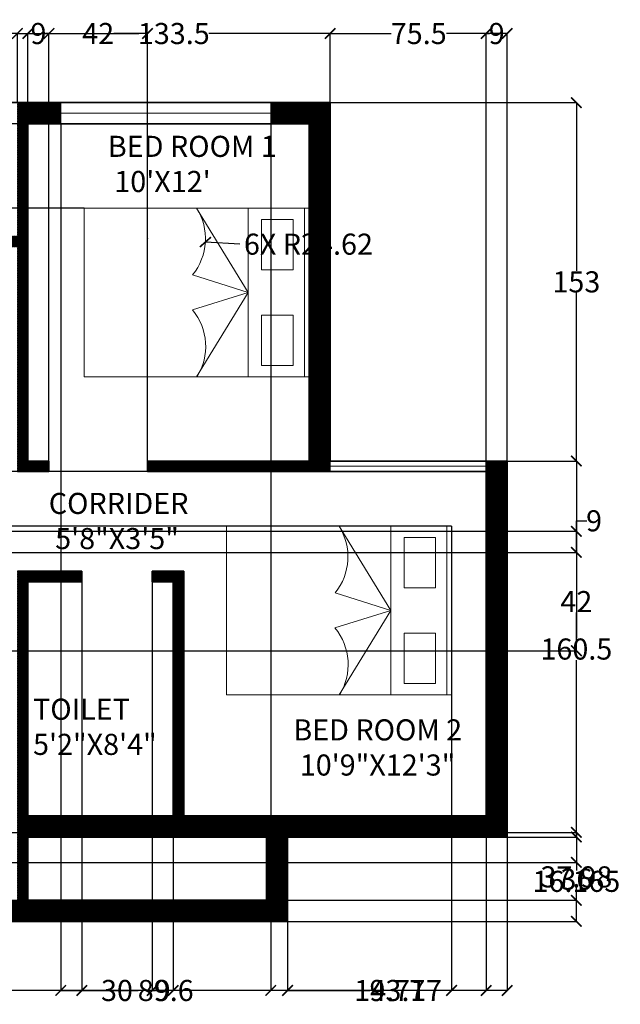
# Model space of a CAD drawing. Units: inches. Extents: x -9 to 675, y 146 to 566.
# Tile 4 of 4: x 418 to 675, y 146 to 566. Entities that reach past the tile are written whole.
import ezdxf

# ---------------------------------------------------------------- set-up
doc = ezdxf.new("R2010")
doc.units = ezdxf.units.IN
doc.header["$MEASUREMENT"] = 0
for name, color, linetype, lineweight in [('A-ANNO-DIMS', 2, 'Continuous', 18), ('A-AREA-IDEN', 7, 'Continuous', 18), ('A-FURN', 8, 'Continuous', 18), ('A-GLAZ', 4, 'Continuous', 18), ('A-WALL', 7, 'Continuous', 35), ('A-WALL-PATT', 252, 'Continuous', 13)]:
    doc.layers.add(name, color=color, linetype=linetype, lineweight=lineweight)
doc.styles.get("Standard").update_dxf_attribs({"font": 'arial.ttf'})
doc.dimstyles.get("Standard").update_dxf_attribs({"dimtxt": 9, "dimasz": 4.5, "dimexe": 0.18, "dimexo": 0.0625, "dimgap": 0.09, "dimtad": 0, "dimtih": 1, "dimtoh": 1, "dimdec": 1, "dimzin": 0, "dimdsep": 46, "dimlunit": 4, "dimtxsty": 'Standard', "dimblk": 'ARCHTICK', "dimcen": 0.09, "dimadec": 0, "dimazin": 0, "dimtfac": 1, "dimtdec": 1, "dimtofl": 0, "dimtmove": 0, "dimatfit": 3, "dimfxl": 1, "dimtolj": 1, "dimtzin": 0, "dimarcsym": 0})

# ---------------------------------------------------------------- blocks, each defined once
blk = doc.blocks.new('BED-DOUBLE-72X96')
for p, q in [((0, 0.1), (0, 72.1)), ((0, 72.1), (96, 72.1)), ((70, 36.1), (48, 72.1)), ((70, 72.1), (70, 0.1)), ((94, 72.1), (94, 0.1)), ((96, 72.1), (96, 0.1)), ((46.29, 43.57), (70, 36.1)), ((70, 36.1), (46.22, 28.65)), ((48, 0.1), (70, 36.1)), ((96, 0.1), (0, 0.1))]:
    blk.add_line(p, q)
for points in [[(89.14, 67.27), (89.14, 45.76), (75.68, 45.76), (75.68, 67.27)], [(89.14, 4.92), (89.14, 26.43), (75.68, 26.43), (75.68, 4.92)]]:
    blk.add_lwpolyline(points, close=True)
for centre, start, end in [((27.13, 59.03), 321.0858, 32.0518), ((27.23, 12.97), 328.2029, 39.5369)]:
    blk.add_arc(centre, 24.62, start, end)
blk = doc.blocks.new('_ArchTick')
at = {"color": 0, "linetype": 'ByBlock', "const_width": 0.15}
blk.add_lwpolyline([(-0.5, -0.5), (0.5, 0.5)], dxfattribs=at)
blk = doc.blocks.new('*D8')
at = {"layer": 'A-ANNO-DIMS', "color": 0, "lineweight": -2, "transparency": 16777216}
for p, q in [((626.3, 217.45), (626.3, 151.83)), ((39.3, 181.45), (39.3, 151.83)), ((39.3, 152.01), (322.77, 152.01)), ((626.3, 152.01), (342.83, 152.01))]:
    blk.add_line(p, q, dxfattribs=at)
at = {"layer": 'Defpoints', "color": 0, "transparency": 16777216}
for p in [(626.3, 217.51), (39.3, 181.51), (626.3, 152.01)]:
    blk.add_point(p, dxfattribs=at)
at = {"layer": 'A-ANNO-DIMS', "color": 0, "lineweight": -2, "transparency": 16777216, "xscale": 4.5, "yscale": 4.5, "zscale": 4.5, "rotation": 180}
blk.add_blockref('_ArchTick', (39.3, 152.01), dxfattribs=at)
at = {"layer": 'A-ANNO-DIMS', "color": 0, "lineweight": -2, "transparency": 16777216, "xscale": 4.5, "yscale": 4.5, "zscale": 4.5}
blk.add_blockref('_ArchTick', (626.3, 152.01), dxfattribs=at)
at = {"layer": 'A-ANNO-DIMS', "color": 0, "transparency": 16777216, "insert": (332.8, 152.01), "char_height": 9, "attachment_point": 5}
blk.add_mtext('\\A1;587', dxfattribs=at)
blk = doc.blocks.new('*D13')
at = {"layer": 'A-ANNO-DIMS', "color": 0, "lineweight": -2, "transparency": 16777216}
for p, q in [((286.8, 531.07), (286.8, 560.69)), ((286.8, 560.51), (337.17, 560.51)), ((417.3, 560.51), (366.94, 560.51)), ((417.3, 531.07), (417.3, 560.69))]:
    blk.add_line(p, q, dxfattribs=at)
at = {"layer": 'Defpoints', "color": 0, "transparency": 16777216}
for p in [(417.3, 560.51), (286.8, 531.01), (417.3, 531.01)]:
    blk.add_point(p, dxfattribs=at)
at = {"layer": 'A-ANNO-DIMS', "color": 0, "lineweight": -2, "transparency": 16777216, "xscale": 4.5, "yscale": 4.5, "zscale": 4.5, "rotation": 180}
blk.add_blockref('_ArchTick', (286.8, 560.51), dxfattribs=at)
at = {"layer": 'A-ANNO-DIMS', "color": 0, "lineweight": -2, "transparency": 16777216, "xscale": 4.5, "yscale": 4.5, "zscale": 4.5}
blk.add_blockref('_ArchTick', (417.3, 560.51), dxfattribs=at)
at = {"layer": 'A-ANNO-DIMS', "color": 0, "transparency": 16777216, "insert": (352.05, 560.51), "char_height": 9, "attachment_point": 5}
blk.add_mtext('\\A1;130.5', dxfattribs=at)
blk = doc.blocks.new('*D14')
at = {"layer": 'A-ANNO-DIMS', "color": 0, "lineweight": -2, "transparency": 16777216}
for p, q in [((417.3, 531.07), (417.3, 560.69)), ((417.3, 560.51), (469.17, 560.51)), ((550.8, 560.51), (498.94, 560.51)), ((550.8, 531.07), (550.8, 560.69))]:
    blk.add_line(p, q, dxfattribs=at)
at = {"layer": 'Defpoints', "color": 0, "transparency": 16777216}
for p in [(550.8, 560.51), (417.3, 531.01), (550.8, 531.01)]:
    blk.add_point(p, dxfattribs=at)
at = {"layer": 'A-ANNO-DIMS', "color": 0, "lineweight": -2, "transparency": 16777216, "xscale": 4.5, "yscale": 4.5, "zscale": 4.5, "rotation": 180}
blk.add_blockref('_ArchTick', (417.3, 560.51), dxfattribs=at)
at = {"layer": 'A-ANNO-DIMS', "color": 0, "lineweight": -2, "transparency": 16777216, "xscale": 4.5, "yscale": 4.5, "zscale": 4.5}
blk.add_blockref('_ArchTick', (550.8, 560.51), dxfattribs=at)
at = {"layer": 'A-ANNO-DIMS', "color": 0, "transparency": 16777216, "insert": (484.05, 560.51), "char_height": 9, "attachment_point": 5}
blk.add_mtext('\\A1;133.5', dxfattribs=at)
blk = doc.blocks.new('*D15')
at = {"layer": 'A-ANNO-DIMS', "color": 0, "lineweight": -2, "transparency": 16777216}
for p, q in [((550.8, 378.07), (550.8, 560.69)), ((550.8, 560.51), (576.78, 560.51)), ((626.3, 560.51), (600.33, 560.51)), ((626.3, 378.07), (626.3, 560.69))]:
    blk.add_line(p, q, dxfattribs=at)
at = {"layer": 'Defpoints', "color": 0, "transparency": 16777216}
for p in [(626.3, 560.51), (550.8, 378.01), (626.3, 378.01)]:
    blk.add_point(p, dxfattribs=at)
at = {"layer": 'A-ANNO-DIMS', "color": 0, "lineweight": -2, "transparency": 16777216, "xscale": 4.5, "yscale": 4.5, "zscale": 4.5, "rotation": 180}
blk.add_blockref('_ArchTick', (550.8, 560.51), dxfattribs=at)
at = {"layer": 'A-ANNO-DIMS', "color": 0, "lineweight": -2, "transparency": 16777216, "xscale": 4.5, "yscale": 4.5, "zscale": 4.5}
blk.add_blockref('_ArchTick', (626.3, 560.51), dxfattribs=at)
at = {"layer": 'A-ANNO-DIMS', "color": 0, "transparency": 16777216, "insert": (588.55, 560.51), "char_height": 9, "attachment_point": 5}
blk.add_mtext('\\A1;75.5', dxfattribs=at)
blk = doc.blocks.new('*D18')
at = {"layer": 'A-ANNO-DIMS', "color": 0, "lineweight": -2, "transparency": 16777216}
for p, q in [((550.87, 531.01), (655.98, 531.01)), ((655.8, 531.01), (655.8, 459.2)), ((655.8, 378.01), (655.8, 449.82)), ((550.87, 378.01), (655.98, 378.01))]:
    blk.add_line(p, q, dxfattribs=at)
at = {"layer": 'Defpoints', "color": 0, "transparency": 16777216}
for p in [(550.8, 531.01), (655.8, 531.01), (550.8, 378.01)]:
    blk.add_point(p, dxfattribs=at)
at = {"layer": 'A-ANNO-DIMS', "color": 0, "lineweight": -2, "transparency": 16777216, "xscale": 4.5, "yscale": 4.5, "zscale": 4.5}
for p, rotation in [((655.8, 531.01), 90), ((655.8, 378.01), 270)]:
    blk.add_blockref('_ArchTick', p, dxfattribs=dict(at, rotation=rotation))
at = {"layer": 'A-ANNO-DIMS', "color": 0, "transparency": 16777216, "insert": (655.8, 454.51), "char_height": 9, "attachment_point": 5}
blk.add_mtext('\\A1;153', dxfattribs=at)
blk = doc.blocks.new('*D19')
at = {"layer": 'A-ANNO-DIMS', "color": 0, "lineweight": -2, "transparency": 16777216}
for p, q in [((626.37, 378.01), (655.98, 378.01)), ((655.8, 378.01), (655.8, 302.44)), ((655.8, 217.51), (655.8, 293.07)), ((626.37, 217.51), (655.98, 217.51))]:
    blk.add_line(p, q, dxfattribs=at)
at = {"layer": 'Defpoints', "color": 0, "transparency": 16777216}
for p in [(626.3, 378.01), (655.8, 378.01), (626.3, 217.51)]:
    blk.add_point(p, dxfattribs=at)
at = {"layer": 'A-ANNO-DIMS', "color": 0, "lineweight": -2, "transparency": 16777216, "xscale": 4.5, "yscale": 4.5, "zscale": 4.5}
for p, rotation in [((655.8, 378.01), 90), ((655.8, 217.51), 270)]:
    blk.add_blockref('_ArchTick', p, dxfattribs=dict(at, rotation=rotation))
at = {"layer": 'A-ANNO-DIMS', "color": 0, "transparency": 16777216, "insert": (655.8, 297.76), "char_height": 9, "attachment_point": 5}
blk.add_mtext('\\A1;160.5', dxfattribs=at)
blk = doc.blocks.new('*D21')
at = {"layer": 'A-ANNO-DIMS', "color": 0, "lineweight": -2, "transparency": 16777216}
for p, q in [((532.61, 217.45), (532.61, 151.83)), ((626.3, 217.45), (626.3, 151.83)), ((532.61, 152.01), (567.68, 152.01)), ((626.3, 152.01), (591.23, 152.01))]:
    blk.add_line(p, q, dxfattribs=at)
at = {"layer": 'Defpoints', "color": 0, "transparency": 16777216}
for p in [(532.61, 217.51), (626.3, 217.51), (626.3, 152.01)]:
    blk.add_point(p, dxfattribs=at)
at = {"layer": 'A-ANNO-DIMS', "color": 0, "lineweight": -2, "transparency": 16777216, "xscale": 4.5, "yscale": 4.5, "zscale": 4.5, "rotation": 180}
blk.add_blockref('_ArchTick', (532.61, 152.01), dxfattribs=at)
at = {"layer": 'A-ANNO-DIMS', "color": 0, "lineweight": -2, "transparency": 16777216, "xscale": 4.5, "yscale": 4.5, "zscale": 4.5}
blk.add_blockref('_ArchTick', (626.3, 152.01), dxfattribs=at)
at = {"layer": 'A-ANNO-DIMS', "color": 0, "transparency": 16777216, "insert": (579.46, 152.01), "char_height": 9, "attachment_point": 5}
blk.add_mtext('\\A1;93.7', dxfattribs=at)
blk = doc.blocks.new('*D22')
at = {"layer": 'A-ANNO-DIMS', "color": 0, "lineweight": -2, "transparency": 16777216}
for p, q in [((196.87, 219.49), (655.98, 219.49)), ((655.8, 219.49), (655.8, 205.19)), ((655.8, 181.51), (655.8, 195.81)), ((196.87, 181.51), (655.98, 181.51))]:
    blk.add_line(p, q, dxfattribs=at)
at = {"layer": 'Defpoints', "color": 0, "transparency": 16777216}
for p in [(196.8, 219.49), (655.8, 219.49), (196.8, 181.51)]:
    blk.add_point(p, dxfattribs=at)
at = {"layer": 'A-ANNO-DIMS', "color": 0, "lineweight": -2, "transparency": 16777216, "xscale": 4.5, "yscale": 4.5, "zscale": 4.5}
for p, rotation in [((655.8, 219.49), 90), ((655.8, 181.51), 270)]:
    blk.add_blockref('_ArchTick', p, dxfattribs=dict(at, rotation=rotation))
at = {"layer": 'A-ANNO-DIMS', "color": 0, "transparency": 16777216, "insert": (655.8, 200.5), "char_height": 9, "attachment_point": 5}
blk.add_mtext('\\A1;37.98', dxfattribs=at)
blk = doc.blocks.new('*D23')
at = {"layer": 'A-ANNO-DIMS', "color": 0, "lineweight": -2, "transparency": 16777216}
for p, q in [((532.67, 217.51), (655.98, 217.51)), ((655.8, 217.51), (655.8, 204.2)), ((655.8, 181.51), (655.8, 194.82)), ((532.67, 181.51), (655.98, 181.51))]:
    blk.add_line(p, q, dxfattribs=at)
at = {"layer": 'Defpoints', "color": 0, "transparency": 16777216}
for p in [(532.61, 217.51), (655.8, 217.51), (532.61, 181.51)]:
    blk.add_point(p, dxfattribs=at)
at = {"layer": 'A-ANNO-DIMS', "color": 0, "lineweight": -2, "transparency": 16777216, "xscale": 4.5, "yscale": 4.5, "zscale": 4.5}
for p, rotation in [((655.8, 217.51), 90), ((655.8, 181.51), 270)]:
    blk.add_blockref('_ArchTick', p, dxfattribs=dict(at, rotation=rotation))
at = {"layer": 'A-ANNO-DIMS', "color": 0, "transparency": 16777216, "insert": (655.8, 199.51), "char_height": 9, "attachment_point": 5}
blk.add_mtext('\\A1;36', dxfattribs=at)
blk = doc.blocks.new('*D27')
at = {"layer": 'A-ANNO-DIMS', "color": 0, "lineweight": -2, "transparency": 16777216}
for p, q in [((435.8, 521.95), (435.8, 151.83)), ((525.4, 521.95), (525.4, 151.83)), ((435.8, 152.01), (468.82, 152.01)), ((525.4, 152.01), (492.38, 152.01))]:
    blk.add_line(p, q, dxfattribs=at)
at = {"layer": 'Defpoints', "color": 0, "transparency": 16777216}
for p in [(435.8, 522.01), (525.4, 522.01), (525.4, 152.01)]:
    blk.add_point(p, dxfattribs=at)
at = {"layer": 'A-ANNO-DIMS', "color": 0, "lineweight": -2, "transparency": 16777216, "xscale": 4.5, "yscale": 4.5, "zscale": 4.5, "rotation": 180}
blk.add_blockref('_ArchTick', (435.8, 152.01), dxfattribs=at)
at = {"layer": 'A-ANNO-DIMS', "color": 0, "lineweight": -2, "transparency": 16777216, "xscale": 4.5, "yscale": 4.5, "zscale": 4.5}
blk.add_blockref('_ArchTick', (525.4, 152.01), dxfattribs=at)
at = {"layer": 'A-ANNO-DIMS', "color": 0, "transparency": 16777216, "insert": (480.6, 152.01), "char_height": 9, "attachment_point": 5}
blk.add_mtext('\\A1;89.6', dxfattribs=at)
blk = doc.blocks.new('*D33')
at = {"layer": 'A-ANNO-DIMS', "color": 0, "lineweight": -2, "transparency": 16777216}
for p, q in [((655.8, 348.01), (655.8, 352.51)), ((655.8, 352.51), (660.3, 352.51)), ((196.87, 348.01), (655.98, 348.01)), ((655.8, 339.01), (655.8, 348.01)), ((196.87, 339.01), (655.98, 339.01))]:
    blk.add_line(p, q, dxfattribs=at)
at = {"layer": 'Defpoints', "color": 0, "transparency": 16777216}
for p in [(196.8, 348.01), (655.8, 348.01), (196.8, 339.01)]:
    blk.add_point(p, dxfattribs=at)
at = {"layer": 'A-ANNO-DIMS', "color": 0, "lineweight": -2, "transparency": 16777216, "xscale": 4.5, "yscale": 4.5, "zscale": 4.5}
for p, rotation in [((655.8, 348.01), 90), ((655.8, 339.01), 270)]:
    blk.add_blockref('_ArchTick', p, dxfattribs=dict(at, rotation=rotation))
at = {"layer": 'A-ANNO-DIMS', "color": 0, "transparency": 16777216, "insert": (663.35, 352.51), "char_height": 9, "attachment_point": 5}
blk.add_mtext('\\A1;9', dxfattribs=at)
blk = doc.blocks.new('*D34')
at = {"layer": 'A-ANNO-DIMS', "color": 0, "lineweight": -2, "transparency": 16777216}
for p, q in [((196.87, 339.01), (655.98, 339.01)), ((655.8, 339.01), (655.8, 322.62)), ((655.8, 297.01), (655.8, 313.4)), ((196.87, 297.01), (655.98, 297.01))]:
    blk.add_line(p, q, dxfattribs=at)
at = {"layer": 'Defpoints', "color": 0, "transparency": 16777216}
for p in [(196.8, 339.01), (655.8, 339.01), (196.8, 297.01)]:
    blk.add_point(p, dxfattribs=at)
at = {"layer": 'A-ANNO-DIMS', "color": 0, "lineweight": -2, "transparency": 16777216, "xscale": 4.5, "yscale": 4.5, "zscale": 4.5}
for p, rotation in [((655.8, 339.01), 90), ((655.8, 297.01), 270)]:
    blk.add_blockref('_ArchTick', p, dxfattribs=dict(at, rotation=rotation))
at = {"layer": 'A-ANNO-DIMS', "color": 0, "transparency": 16777216, "insert": (655.8, 318.01), "char_height": 9, "attachment_point": 5}
blk.add_mtext('\\A1;42', dxfattribs=at)
blk = doc.blocks.new('*D35')
at = {"layer": 'A-ANNO-DIMS', "color": 0, "lineweight": -2, "transparency": 16777216}
for p, q in [((421.8, 378.07), (421.8, 560.69)), ((421.8, 560.51), (423.25, 560.51)), ((430.8, 560.51), (429.35, 560.51)), ((430.8, 378.07), (430.8, 560.69))]:
    blk.add_line(p, q, dxfattribs=at)
at = {"layer": 'Defpoints', "color": 0, "transparency": 16777216}
for p in [(430.8, 560.51), (421.8, 378.01), (430.8, 378.01)]:
    blk.add_point(p, dxfattribs=at)
at = {"layer": 'A-ANNO-DIMS', "color": 0, "lineweight": -2, "transparency": 16777216, "xscale": 4.5, "yscale": 4.5, "zscale": 4.5, "rotation": 180}
blk.add_blockref('_ArchTick', (421.8, 560.51), dxfattribs=at)
at = {"layer": 'A-ANNO-DIMS', "color": 0, "lineweight": -2, "transparency": 16777216, "xscale": 4.5, "yscale": 4.5, "zscale": 4.5}
blk.add_blockref('_ArchTick', (430.8, 560.51), dxfattribs=at)
at = {"layer": 'A-ANNO-DIMS', "color": 0, "transparency": 16777216, "insert": (426.3, 560.51), "char_height": 9, "attachment_point": 5}
blk.add_mtext('\\A1;9', dxfattribs=at)
blk = doc.blocks.new('*D36')
at = {"layer": 'A-ANNO-DIMS', "color": 0, "lineweight": -2, "transparency": 16777216}
for p, q in [((430.8, 378.07), (430.8, 560.69)), ((430.8, 560.51), (445.13, 560.51)), ((472.8, 560.51), (458.47, 560.51)), ((472.8, 378.07), (472.8, 560.69))]:
    blk.add_line(p, q, dxfattribs=at)
at = {"layer": 'Defpoints', "color": 0, "transparency": 16777216}
for p in [(472.8, 560.51), (430.8, 378.01), (472.8, 378.01)]:
    blk.add_point(p, dxfattribs=at)
at = {"layer": 'A-ANNO-DIMS', "color": 0, "lineweight": -2, "transparency": 16777216, "xscale": 4.5, "yscale": 4.5, "zscale": 4.5, "rotation": 180}
blk.add_blockref('_ArchTick', (430.8, 560.51), dxfattribs=at)
at = {"layer": 'A-ANNO-DIMS', "color": 0, "lineweight": -2, "transparency": 16777216, "xscale": 4.5, "yscale": 4.5, "zscale": 4.5}
blk.add_blockref('_ArchTick', (472.8, 560.51), dxfattribs=at)
at = {"layer": 'A-ANNO-DIMS', "color": 0, "transparency": 16777216, "insert": (451.8, 560.51), "char_height": 9, "attachment_point": 5}
blk.add_mtext('\\A1;42', dxfattribs=at)
blk = doc.blocks.new('*D37')
at = {"layer": 'A-ANNO-DIMS', "color": 0, "lineweight": -2, "transparency": 16777216}
for p, q in [((444.8, 326.45), (444.8, 151.83)), ((474.8, 326.45), (474.8, 151.83)), ((444.8, 152.01), (453.28, 152.01)), ((474.8, 152.01), (466.32, 152.01))]:
    blk.add_line(p, q, dxfattribs=at)
at = {"layer": 'Defpoints', "color": 0, "transparency": 16777216}
for p in [(444.8, 326.51), (474.8, 326.51), (474.8, 152.01)]:
    blk.add_point(p, dxfattribs=at)
at = {"layer": 'A-ANNO-DIMS', "color": 0, "lineweight": -2, "transparency": 16777216, "xscale": 4.5, "yscale": 4.5, "zscale": 4.5, "rotation": 180}
blk.add_blockref('_ArchTick', (444.8, 152.01), dxfattribs=at)
at = {"layer": 'A-ANNO-DIMS', "color": 0, "lineweight": -2, "transparency": 16777216, "xscale": 4.5, "yscale": 4.5, "zscale": 4.5}
blk.add_blockref('_ArchTick', (474.8, 152.01), dxfattribs=at)
at = {"layer": 'A-ANNO-DIMS', "color": 0, "transparency": 16777216, "insert": (459.8, 152.01), "char_height": 9, "attachment_point": 5}
blk.add_mtext('\\A1;30', dxfattribs=at)
blk = doc.blocks.new('*D38')
at = {"layer": 'A-ANNO-DIMS', "color": 0, "lineweight": -2, "transparency": 16777216}
for p, q in [((474.8, 326.45), (474.8, 151.83)), ((483.8, 326.45), (483.8, 151.83)), ((474.8, 152.01), (476.25, 152.01)), ((483.8, 152.01), (482.35, 152.01))]:
    blk.add_line(p, q, dxfattribs=at)
at = {"layer": 'Defpoints', "color": 0, "transparency": 16777216}
for p in [(474.8, 326.51), (483.8, 326.51), (483.8, 152.01)]:
    blk.add_point(p, dxfattribs=at)
at = {"layer": 'A-ANNO-DIMS', "color": 0, "lineweight": -2, "transparency": 16777216, "xscale": 4.5, "yscale": 4.5, "zscale": 4.5, "rotation": 180}
blk.add_blockref('_ArchTick', (474.8, 152.01), dxfattribs=at)
at = {"layer": 'A-ANNO-DIMS', "color": 0, "lineweight": -2, "transparency": 16777216, "xscale": 4.5, "yscale": 4.5, "zscale": 4.5}
blk.add_blockref('_ArchTick', (483.8, 152.01), dxfattribs=at)
at = {"layer": 'A-ANNO-DIMS', "color": 0, "transparency": 16777216, "insert": (479.3, 152.01), "char_height": 9, "attachment_point": 5}
blk.add_mtext('\\A1;9', dxfattribs=at)
blk = doc.blocks.new('*D45')
at = {"layer": 'A-ANNO-DIMS', "color": 0, "lineweight": -2, "transparency": 16777216}
for p, q in [((80.35, 206.67), (655.98, 206.67)), ((655.8, 206.67), (655.8, 203.28)), ((655.8, 190.51), (655.8, 193.91)), ((48.37, 190.51), (655.98, 190.51))]:
    blk.add_line(p, q, dxfattribs=at)
at = {"layer": 'Defpoints', "color": 0, "transparency": 16777216}
for p in [(80.28, 206.67), (655.8, 206.67), (48.3, 190.51)]:
    blk.add_point(p, dxfattribs=at)
at = {"layer": 'A-ANNO-DIMS', "color": 0, "lineweight": -2, "transparency": 16777216, "xscale": 4.5, "yscale": 4.5, "zscale": 4.5}
for p, rotation in [((655.8, 206.67), 90), ((655.8, 190.51), 270)]:
    blk.add_blockref('_ArchTick', p, dxfattribs=dict(at, rotation=rotation))
at = {"layer": 'A-ANNO-DIMS', "color": 0, "transparency": 16777216, "insert": (655.8, 198.59), "char_height": 9, "attachment_point": 5}
blk.add_mtext('\\A1;16.165', dxfattribs=at)
blk = doc.blocks.new('*D46')
at = {"layer": 'A-ANNO-DIMS', "color": 0, "lineweight": -2, "transparency": 16777216}
for p, q in [((435.74, 522.01), (9.62, 522.01)), ((9.8, 522.01), (9.8, 508.7)), ((9.8, 486.01), (9.8, 499.32)), ((445.74, 486.01), (9.62, 486.01))]:
    blk.add_line(p, q, dxfattribs=at)
at = {"layer": 'Defpoints', "color": 0, "transparency": 16777216}
for p in [(435.8, 522.01), (9.8, 486.01), (445.8, 486.01)]:
    blk.add_point(p, dxfattribs=at)
at = {"layer": 'A-ANNO-DIMS', "color": 0, "lineweight": -2, "transparency": 16777216, "xscale": 4.5, "yscale": 4.5, "zscale": 4.5}
for p, rotation in [((9.8, 522.01), 90), ((9.8, 486.01), 270)]:
    blk.add_blockref('_ArchTick', p, dxfattribs=dict(at, rotation=rotation))
at = {"layer": 'A-ANNO-DIMS', "color": 0, "transparency": 16777216, "insert": (9.8, 504.01), "char_height": 9, "attachment_point": 5}
blk.add_mtext('\\A1;36', dxfattribs=at)
blk = doc.blocks.new('*D47')
at = {"layer": 'A-ANNO-DIMS', "color": 0, "lineweight": -2, "transparency": 16777216}
for p, q in [((617.24, 373.51), (9.62, 373.51)), ((9.8, 373.51), (9.8, 366.56)), ((9.8, 350.24), (9.8, 357.19)), ((602.52, 350.24), (9.62, 350.24))]:
    blk.add_line(p, q, dxfattribs=at)
at = {"layer": 'Defpoints', "color": 0, "transparency": 16777216}
for p in [(617.3, 373.51), (9.8, 350.24), (602.59, 350.24)]:
    blk.add_point(p, dxfattribs=at)
at = {"layer": 'A-ANNO-DIMS', "color": 0, "lineweight": -2, "transparency": 16777216, "xscale": 4.5, "yscale": 4.5, "zscale": 4.5}
for p, rotation in [((9.8, 373.51), 90), ((9.8, 350.24), 270)]:
    blk.add_blockref('_ArchTick', p, dxfattribs=dict(at, rotation=rotation))
at = {"layer": 'A-ANNO-DIMS', "color": 0, "transparency": 16777216, "insert": (9.8, 361.87), "char_height": 9, "attachment_point": 5}
blk.add_mtext('\\A1;23.27', dxfattribs=at)
blk = doc.blocks.new('*D48')
at = {"layer": 'A-ANNO-DIMS', "color": 0, "lineweight": -2, "transparency": 16777216}
for p, q in [((617.3, 373.45), (617.3, 151.83)), ((602.59, 350.18), (602.59, 151.83)), ((602.59, 152.01), (598.09, 152.01)), ((617.3, 152.01), (602.59, 152.01))]:
    blk.add_line(p, q, dxfattribs=at)
at = {"layer": 'Defpoints', "color": 0, "transparency": 16777216}
for p in [(617.3, 373.51), (602.59, 350.24), (602.59, 152.01)]:
    blk.add_point(p, dxfattribs=at)
at = {"layer": 'A-ANNO-DIMS', "color": 0, "lineweight": -2, "transparency": 16777216, "xscale": 4.5, "yscale": 4.5, "zscale": 4.5, "rotation": 180}
blk.add_blockref('_ArchTick', (602.59, 152.01), dxfattribs=at)
at = {"layer": 'A-ANNO-DIMS', "color": 0, "lineweight": -2, "transparency": 16777216, "xscale": 4.5, "yscale": 4.5, "zscale": 4.5}
blk.add_blockref('_ArchTick', (617.3, 152.01), dxfattribs=at)
at = {"layer": 'A-ANNO-DIMS', "color": 0, "transparency": 16777216, "insert": (579.74, 152.01), "char_height": 9, "attachment_point": 5}
blk.add_mtext('\\A1;14.717', dxfattribs=at)
blk = doc.blocks.new('*D49')
at = {"layer": 'A-ANNO-DIMS', "color": 0, "lineweight": -2, "transparency": 16777216}
for p, q in [((617.3, 226.57), (617.3, 560.69)), ((617.3, 560.51), (618.75, 560.51)), ((626.3, 560.51), (624.85, 560.51)), ((626.3, 217.57), (626.3, 560.69))]:
    blk.add_line(p, q, dxfattribs=at)
at = {"layer": 'Defpoints', "color": 0, "transparency": 16777216}
for p in [(626.3, 560.51), (617.3, 226.51), (626.3, 217.51)]:
    blk.add_point(p, dxfattribs=at)
at = {"layer": 'A-ANNO-DIMS', "color": 0, "lineweight": -2, "transparency": 16777216, "xscale": 4.5, "yscale": 4.5, "zscale": 4.5, "rotation": 180}
blk.add_blockref('_ArchTick', (617.3, 560.51), dxfattribs=at)
at = {"layer": 'A-ANNO-DIMS', "color": 0, "lineweight": -2, "transparency": 16777216, "xscale": 4.5, "yscale": 4.5, "zscale": 4.5}
blk.add_blockref('_ArchTick', (626.3, 560.51), dxfattribs=at)
at = {"layer": 'A-ANNO-DIMS', "color": 0, "transparency": 16777216, "insert": (621.8, 560.51), "char_height": 9, "attachment_point": 5}
blk.add_mtext('\\A1;9', dxfattribs=at)
blk = doc.blocks.new('*D57')
at = {"layer": 'A-ANNO-DIMS', "color": 0, "lineweight": -2, "transparency": 16777216}
for p, q in [((472.84, 472.94), (473.02, 472.94)), ((472.93, 472.85), (472.93, 473.03)), ((512.26, 470.59), (497.51, 471.47))]:
    blk.add_line(p, q, dxfattribs=at)
at = {"layer": 'Defpoints', "color": 0, "transparency": 16777216}
for p in [(472.93, 472.94), (497.51, 471.47)]:
    blk.add_point(p, dxfattribs=at)
at = {"layer": 'A-ANNO-DIMS', "color": 0, "lineweight": -2, "transparency": 16777216, "xscale": 4.5, "yscale": 4.5, "zscale": 4.5, "rotation": 176.5680660431025}
blk.add_blockref('_ArchTick', (497.51, 471.47), dxfattribs=at)
at = {"layer": 'A-ANNO-DIMS', "color": 0, "transparency": 16777216, "insert": (541.49, 470.59), "char_height": 9, "attachment_point": 5}
blk.add_mtext('\\A1;6X R24.62', dxfattribs=at)

msp = doc.modelspace()

# ---------------------------------------------------------------- hatches: boundary and pattern name
at = {"layer": 'A-WALL-PATT'}
h = msp.add_hatch(dxfattribs=at)
h.set_pattern_fill('ANSI31', color=256)
h.paths.add_polyline_path([(361.8026, 244.5097), (357.3026, 244.5097), (357.3026, 228.4917), (286.8026, 228.4917), (196.8026, 228.4917), (196.8026, 297.0097), (192.3026, 297.0097), (192.3026, 190.5097), (196.8026, 190.5097), (196.8026, 219.4917), (286.8026, 219.4917), (357.3026, 219.4917), (357.3026, 217.5097), (357.3026, 214.9917), (361.8026, 214.9917), (361.8026, 217.5097)])
h.paths.add_polyline_path([(532.6092, 217.5097), (541.8026, 217.5097), (550.8026, 217.5097), (626.3026, 217.5097), (626.3026, 373.5097), (626.3026, 378.0097), (617.3026, 378.0097), (617.3026, 373.5097), (617.3026, 226.5097), (550.8026, 226.5097), (541.8026, 226.5097), (488.3026, 226.5097), (488.3026, 331.0097), (483.8026, 331.0097), (474.8026, 331.0097), (474.8026, 326.5097), (483.8026, 326.5097), (483.8026, 226.5097), (421.8026, 226.5097), (421.8026, 326.5097), (444.8026, 326.5097), (444.8026, 331.0097), (421.8026, 331.0097), (417.3026, 331.0097), (417.3026, 217.5097), (417.3026, 190.5097), (387.6027, 190.5097), (361.8026, 190.5097), (361.8026, 195.0097), (357.3026, 195.0097), (357.3026, 190.5097), (357.3026, 181.5097), (387.6027, 181.5097), (421.8026, 181.5097), (532.6092, 181.5097)])
h.paths.add_polyline_path([(421.8026, 190.5097), (421.8026, 217.5097), (523.6092, 217.5097), (523.6092, 190.5097)], flags=16)
h.paths.add_polyline_path([(550.8026, 378.0097), (550.8026, 531.0097), (525.3955, 531.0097), (525.3955, 522.0097), (541.8026, 522.0097), (541.8026, 378.0097), (472.8026, 378.0097), (472.8026, 373.5097), (483.8026, 373.5097), (488.3026, 373.5097), (541.8026, 373.5097), (550.8026, 373.5097)])
h.paths.add_polyline_path([(130.3026, 469.5097), (146.3026, 469.5097), (146.3026, 474.0097), (130.3026, 474.0097), (130.3026, 522.0097), (143.3026, 522.0097), (143.3026, 531.0097), (121.3026, 531.0097), (121.3026, 351.7597), (121.3026, 348.0097), (130.3026, 348.0097), (139.3026, 348.0097), (139.3026, 351.7597), (130.3026, 351.7597)])
h.paths.add_polyline_path([(211.9624, 531.0097), (179.3026, 531.0097), (179.3026, 522.0097), (192.3026, 522.0097), (192.3026, 474.0097), (176.3026, 474.0097), (176.3026, 469.5097), (192.3026, 469.5097), (192.3026, 351.7597), (169.3026, 351.7597), (169.3026, 348.0097), (192.3026, 348.0097), (192.3026, 339.0097), (196.8026, 339.0097), (196.8026, 348.0097), (226.8026, 348.0097), (226.8026, 352.5097), (196.8026, 352.5097), (196.8026, 469.5097), (226.8026, 469.5097), (226.8026, 474.0097), (196.8026, 474.0097), (196.8026, 522.0097), (211.9624, 522.0097)])
h.paths.add_polyline_path([(291.3026, 522.0097), (291.3026, 531.0097), (286.8026, 531.0097), (286.8026, 522.0097), (286.8026, 352.5097), (256.8026, 352.5097), (256.8026, 348.0097), (286.8026, 348.0097), (286.8026, 346.5097), (291.3026, 346.5097)])
h.paths.add_polyline_path([(417.3026, 474.0097), (291.3026, 474.0097), (291.3026, 469.5097), (417.3026, 469.5097)])
h.paths.add_polyline_path([(421.8026, 522.0097), (435.8002, 522.0097), (435.8002, 531.0097), (417.3026, 531.0097), (417.3026, 522.0097), (417.3026, 373.5097), (421.8026, 373.5097), (430.8026, 373.5097), (430.8026, 378.0097), (421.8026, 378.0097)])
h.paths.add_polyline_path([(48.3026, 348.0097), (48.3026, 351.7597), (39.3026, 351.7597), (39.3026, 348.0097), (39.3026, 181.5097), (121.3026, 181.5097), (196.8026, 181.5097), (196.8026, 190.5097), (192.3026, 190.5097), (121.3026, 190.5097), (48.3026, 190.5097)])

# ---------------------------------------------------------------- linework, layer by layer
at = {"layer": 'A-GLAZ'}
for p, q in [((435.8002, 531.0097), (435.8002, 522.0097)), ((525.3955, 531.0097), (525.3955, 522.0097)), ((435.8002, 526.5097), (525.3955, 526.5097)), ((550.8026, 378.0097), (550.8026, 373.5097)), ((550.8026, 375.7597), (617.3026, 375.7597)), ((617.3026, 373.5097), (617.3026, 378.0097))]:
    msp.add_line(p, q, dxfattribs=at)
at = {"layer": 'A-WALL'}
for p, q in [((121.3026, 531.0097), (550.8026, 531.0097)), ((550.8026, 531.0097), (550.8026, 378.0097)), ((421.8026, 522.0097), (421.8026, 378.0097)), ((421.8026, 522.0097), (541.8026, 522.0097)), ((541.8026, 522.0097), (541.8026, 378.0097)), ((421.8026, 378.0097), (430.8026, 378.0097)), ((430.8026, 378.0097), (430.8026, 373.5097)), ((472.8026, 378.0097), (472.8026, 373.5097)), ((472.8026, 378.0097), (541.8026, 378.0097)), ((550.8026, 378.0097), (626.3026, 378.0097)), ((626.3026, 373.5097), (626.3026, 378.0097)), ((421.8026, 373.5097), (417.3026, 373.5097)), ((421.8026, 373.5097), (430.8026, 373.5097)), ((472.8026, 373.5097), (483.8026, 373.5097)), ((488.3026, 373.5097), (483.8026, 373.5097)), ((488.3026, 373.5097), (541.8026, 373.5097)), ((541.8026, 373.5097), (550.8026, 373.5097)), ((550.8026, 373.5097), (617.3026, 373.5097)), ((617.3026, 373.5097), (617.3026, 226.5097)), ((626.3026, 373.5097), (626.3026, 217.5097)), ((421.8026, 331.0097), (417.3026, 331.0097)), ((421.8026, 331.0097), (444.8026, 331.0097)), ((444.8026, 326.5097), (444.8026, 331.0097)), ((474.8026, 326.5097), (474.8026, 331.0097)), ((474.8026, 331.0097), (483.8026, 331.0097)), ((483.8026, 331.0097), (488.3026, 331.0097)), ((488.3026, 331.0097), (488.3026, 226.5097)), ((421.8026, 326.5097), (421.8026, 226.5097)), ((421.8026, 326.5097), (444.8026, 326.5097)), ((474.8026, 326.5097), (483.8026, 326.5097)), ((483.8026, 326.5097), (483.8026, 226.5097)), ((421.8026, 226.5097), (483.8026, 226.5097)), ((488.3026, 226.5097), (541.8026, 226.5097)), ((541.8026, 226.5097), (550.8026, 226.5097)), ((550.8026, 226.5097), (617.3026, 226.5097)), ((421.8026, 217.5097), (523.6092, 217.5097)), ((421.8026, 217.5097), (421.8026, 190.5097)), ((523.6092, 217.5097), (523.6092, 190.5097)), ((532.6092, 217.5097), (532.6092, 181.5097)), ((532.6092, 217.5097), (541.8026, 217.5097)), ((541.8026, 217.5097), (550.8026, 217.5097)), ((550.8026, 217.5097), (626.3026, 217.5097)), ((421.8026, 190.5097), (523.6092, 190.5097)), ((421.8026, 181.5097), (387.6027, 181.5097)), ((421.8026, 181.5097), (532.6092, 181.5097))]:
    msp.add_line(p, q, dxfattribs=at)

# ---------------------------------------------------------------- block references
at = {"layer": 'A-FURN'}
for p in [(445.803, 413.912), (506.586, 278.1398)]:
    msp.add_blockref('BED-DOUBLE-72X96', p, dxfattribs=at)

# ---------------------------------------------------------------- texts
at = {"layer": 'A-AREA-IDEN', "char_height": 9, "attachment_point": 1}
for s, insert in [("BED ROOM 1\\P 10'X12'", (455.9151, 516.8465)), ('CORRIDER\\P 5\'8"X3\'5"', (430.6989, 364.4269)), ('  TOILET\\P  5\'2"X8\'4"', (418.5054, 276.5697)), ('BED ROOM 2\\P 10\'9"X12\'3"', (535.0308, 267.7536))]:
    msp.add_mtext_dynamic_manual_height_columns(s, width=552.217276, gutter_width=1, heights=[0], dxfattribs=dict(at, insert=insert))

# ---------------------------------------------------------------- dimensions: what is measured, and where the dimension line sits
at = {"layer": 'A-ANNO-DIMS'}
for base, p1, p2, override, picture, middle in [((417.3026, 560.5097), (286.8026, 531.0097), (417.3026, 531.0097), {"dimdec": 1, "dimlfac": 1, "dimrnd": 0, "dimzin": 0, "dimdsep": 46, "dimlunit": 2}, '*D13', (352.0526, 560.5097)), ((550.8026, 560.5097), (417.3026, 531.0097), (550.8026, 531.0097), {"dimdec": 1, "dimlfac": 1, "dimrnd": 0, "dimzin": 0, "dimdsep": 46, "dimlunit": 2}, '*D14', (484.0526, 560.5097)), ((430.8026, 560.5097), (421.8026, 378.0097), (430.8026, 378.0097), {"dimdec": 0, "dimlfac": 1, "dimrnd": 0, "dimzin": 0, "dimdsep": 46, "dimlunit": 2}, '*D35', (426.3026, 560.5097)), ((472.8026, 560.5097), (430.8026, 378.0097), (472.8026, 378.0097), {"dimdec": 0, "dimlfac": 1, "dimrnd": 0, "dimzin": 0, "dimdsep": 46, "dimlunit": 2}, '*D36', (451.8026, 560.5097)), ((626.3026, 560.5097), (550.8026, 378.0097), (626.3026, 378.0097), {"dimdec": 1, "dimlfac": 1, "dimrnd": 0, "dimzin": 0, "dimdsep": 46, "dimlunit": 2}, '*D15', (588.5526, 560.5097)), ((626.3026, 560.5097), (617.3026, 226.5097), (626.3026, 217.5097), {"dimdec": 0, "dimlfac": 1, "dimrnd": 0, "dimzin": 0, "dimdsep": 46, "dimlunit": 2}, '*D49', (621.8026, 560.5097)), ((525.3955, 152.0097), (435.8002, 522.0097), (525.3955, 522.0097), {"dimdec": 1, "dimlfac": 1, "dimrnd": 0, "dimzin": 0, "dimdsep": 46, "dimlunit": 2}, '*D27', (480.5979, 152.0097)), ((602.5856, 152.0097), (617.3026, 373.5097), (602.5856, 350.2376), {"dimdec": 3, "dimlfac": 1, "dimrnd": 0, "dimzin": 0, "dimdsep": 46, "dimlunit": 2}, '*D48', (579.7378, 152.0097)), ((474.8026, 152.0097), (444.8026, 326.5097), (474.8026, 326.5097), {"dimdec": 0, "dimlfac": 1, "dimrnd": 0, "dimzin": 0, "dimdsep": 46, "dimlunit": 2}, '*D37', (459.8026, 152.0097)), ((483.8026, 152.0097), (474.8026, 326.5097), (483.8026, 326.5097), {"dimdec": 0, "dimlfac": 1, "dimrnd": 0, "dimzin": 0, "dimdsep": 46, "dimlunit": 2}, '*D38', (479.3026, 152.0097)), ((626.3026, 152.0097), (39.3026, 181.5097), (626.3026, 217.5097), {"dimdec": 0, "dimlfac": 1, "dimrnd": 0, "dimzin": 0, "dimdsep": 46, "dimlunit": 2}, '*D8', (332.8026, 152.0097)), ((626.3026, 152.0097), (532.6092, 217.5097), (626.3026, 217.5097), {"dimdec": 1, "dimlfac": 1, "dimrnd": 0, "dimzin": 0, "dimdsep": 46, "dimlunit": 2}, '*D21', (579.4559, 152.0097))]:
    dim = msp.add_linear_dim(base=base, p1=p1, p2=p2, dimstyle='Standard', override=override, dxfattribs=at)
    dim.commit()
    dim.dimension.update_dxf_attribs({"geometry": picture, "text_midpoint": middle})
for base, p1, p2, override, picture, middle in [((655.8026, 531.0097), (550.8026, 378.0097), (550.8026, 531.0097), {"dimdec": 0, "dimlfac": 1, "dimrnd": 0, "dimzin": 0, "dimdsep": 46, "dimlunit": 2}, '*D18', (655.8026, 454.5097)), ((9.8026, 486.0097), (435.8002, 522.0097), (445.8026, 486.0097), {"dimdec": 0, "dimlfac": 1, "dimrnd": 0, "dimzin": 0, "dimdsep": 46, "dimlunit": 2}, '*D46', (9.8026, 504.0097)), ((655.8026, 378.0097), (626.3026, 217.5097), (626.3026, 378.0097), {"dimdec": 1, "dimlfac": 1, "dimrnd": 0, "dimzin": 0, "dimdsep": 46, "dimlunit": 2}, '*D19', (655.8026, 297.7597)), ((9.8026, 350.2376), (617.3026, 373.5097), (602.5856, 350.2376), {"dimdec": 2, "dimlfac": 1, "dimrnd": 0, "dimzin": 0, "dimdsep": 46, "dimlunit": 2}, '*D47', (9.8026, 361.8737)), ((655.8026, 348.0097), (196.8026, 339.0097), (196.8026, 348.0097), {"dimdec": 0, "dimlfac": 1, "dimrnd": 0, "dimzin": 0, "dimdsep": 46, "dimlunit": 2}, '*D33', (663.3517, 352.5097)), ((655.8026, 339.0097), (196.8026, 297.0097), (196.8026, 339.0097), {"dimdec": 0, "dimlfac": 1, "dimrnd": 0, "dimzin": 0, "dimdsep": 46, "dimlunit": 2}, '*D34', (655.8026, 318.0097)), ((655.8026, 219.4917), (196.8026, 181.5097), (196.8026, 219.4917), {"dimdec": 2, "dimlfac": 1, "dimrnd": 0, "dimzin": 0, "dimdsep": 46, "dimlunit": 2}, '*D22', (655.8026, 200.5007)), ((655.8026, 217.5097), (532.6092, 181.5097), (532.6092, 217.5097), {"dimdec": 0, "dimlfac": 1, "dimrnd": 0, "dimzin": 0, "dimdsep": 46, "dimlunit": 2}, '*D23', (655.8026, 199.5097)), ((655.8026, 206.6747), (48.3026, 190.5097), (80.2837, 206.6747), {"dimdec": 3, "dimlfac": 1, "dimrnd": 0, "dimzin": 0, "dimdsep": 46, "dimlunit": 2}, '*D45', (655.8026, 198.5922))]:
    dim = msp.add_linear_dim(base=base, p1=p1, p2=p2, angle=90, dimstyle='Standard', override=override, dxfattribs=at)
    dim.commit()
    dim.dimension.update_dxf_attribs({"geometry": picture, "text_midpoint": middle})
dim = msp.add_radius_dim(center=(472.9348, 472.9438), mpoint=(497.5114, 471.47), text='6X <>', dimstyle='Standard', override={"dimdec": 2, "dimlfac": 1, "dimrnd": 0, "dimzin": 0, "dimdsep": 46, "dimlunit": 2}, dxfattribs=at)
dim.commit()
dim.dimension.update_dxf_attribs({"geometry": '*D57', "text_midpoint": (512.2574, 470.5857), "dimtype": 164})

doc.saveas('drawing.dxf')
